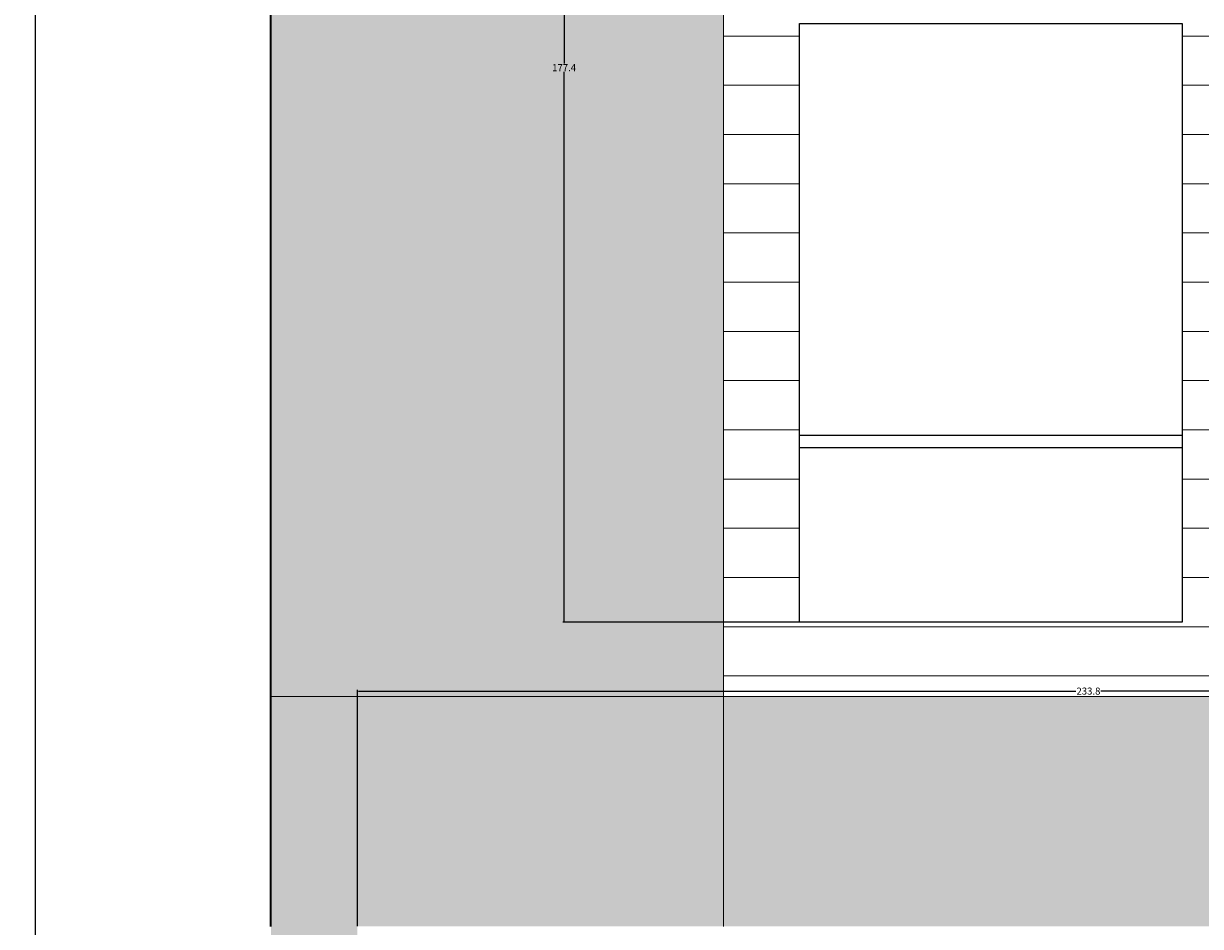
# Model space of a CAD drawing. Units: inches. Extents: x 8 to 634, y 41 to 867.
# Tile 3 of 21: x 8 to 196, y 236 to 380. Entities that reach past the tile are written whole.
import ezdxf

# ---------------------------------------------------------------- set-up
doc = ezdxf.new("R2010")
doc.units = ezdxf.units.IN
doc.header["$MEASUREMENT"] = 0
for name, color, linetype, lineweight in [('A-ANNO-DIMS', 2, 'Continuous', 18), ('A-GLAZ', 4, 'Continuous', 25), ('A-WALL', 7, 'Continuous', 35), ('A-WALL-PANL', 7, 'Continuous', 18), ('A-WALL-PATT', 8, 'Continuous', 9)]:
    doc.layers.add(name, color=color, linetype=linetype, lineweight=lineweight)
doc.styles.get("Standard").update_dxf_attribs({"font": 'arial.ttf'})
doc.dimstyles.get("Standard").update_dxf_attribs({"dimtxt": 1.125, "dimasz": 0.18, "dimexe": 0.18, "dimexo": 0.0625, "dimgap": 0.09, "dimtad": 0, "dimtih": 1, "dimtoh": 1, "dimdec": 4, "dimzin": 0, "dimdsep": 46, "dimlunit": 4, "dimtxsty": 'Standard', "dimcen": 0.09, "dimadec": 0, "dimazin": 0, "dimtfac": 1, "dimtdec": 4, "dimtofl": 0, "dimtmove": 0, "dimatfit": 3, "dimfxl": 1, "dimtolj": 1, "dimtzin": 0, "dimarcsym": 0})

# ---------------------------------------------------------------- blocks, each defined once
blk = doc.blocks.new('WIN-DOUBLE-RAIL')
for p, q in [((0, 29.93), (61.23, 29.93)), ((0, 27.93), (61.23, 27.93))]:
    blk.add_line(p, q)
blk.add_lwpolyline([(0, 95.77), (61.23, 95.77), (61.23, 0), (0, 0)], close=True)
blk = doc.blocks.new('*D20')
at = {"layer": 'A-ANNO-DIMS', "color": 0, "lineweight": -2, "transparency": 16777216}
for p, q in [((144.29, 828.98), (9.51, 828.98)), ((9.69, 828.8), (9.69, 454.93)), ((9.69, 79.74), (9.69, 453.6)), ((47.28, 79.56), (9.51, 79.56))]:
    blk.add_line(p, q, dxfattribs=at)
at = {"layer": 'A-ANNO-DIMS', "color": 0, "transparency": 16777216}
for points in [[(9.66, 828.8), (9.72, 828.8), (9.69, 828.98)], [(9.66, 79.74), (9.72, 79.74), (9.69, 79.56)]]:
    blk.add_solid(points, dxfattribs=at)
at = {"layer": 'Defpoints', "color": 0, "transparency": 16777216}
for p in [(9.69, 828.98), (144.36, 828.98), (47.34, 79.56)]:
    blk.add_point(p, dxfattribs=at)
at = {"layer": 'A-ANNO-DIMS', "color": 0, "transparency": 16777216, "insert": (9.69, 454.27), "char_height": 1.125, "attachment_point": 5}
blk.add_mtext('\\A1;749.4', dxfattribs=at)
blk = doc.blocks.new('*D43')
at = {"layer": 'A-ANNO-DIMS', "color": 0, "lineweight": -2, "transparency": 16777216}
for p, q in [((131.81, 461.65), (94.05, 461.65)), ((94.23, 461.47), (94.23, 373.6)), ((94.23, 284.42), (94.23, 372.29)), ((131.81, 284.24), (94.05, 284.24))]:
    blk.add_line(p, q, dxfattribs=at)
at = {"layer": 'A-ANNO-DIMS', "color": 0, "transparency": 16777216}
for points in [[(94.2, 461.47), (94.26, 461.47), (94.23, 461.65)], [(94.2, 284.42), (94.26, 284.42), (94.23, 284.24)]]:
    blk.add_solid(points, dxfattribs=at)
at = {"layer": 'Defpoints', "color": 0, "transparency": 16777216}
for p in [(94.23, 461.65), (131.88, 461.65), (131.88, 284.24)]:
    blk.add_point(p, dxfattribs=at)
at = {"layer": 'A-ANNO-DIMS', "color": 0, "transparency": 16777216, "insert": (94.23, 372.95), "char_height": 1.125, "attachment_point": 5}
blk.add_mtext('\\A1;177.4', dxfattribs=at)
blk = doc.blocks.new('*D65')
at = {"layer": 'A-ANNO-DIMS', "color": 0, "lineweight": -2, "transparency": 16777216}
for p, q in [((61.18, 235.62), (61.18, 273.39)), ((61.36, 273.21), (176.09, 273.21)), ((294.82, 273.21), (180.09, 273.21)), ((295, 235.62), (295, 273.39))]:
    blk.add_line(p, q, dxfattribs=at)
at = {"layer": 'A-ANNO-DIMS', "color": 0, "transparency": 16777216}
for points in [[(61.36, 273.24), (61.36, 273.18), (61.18, 273.21)], [(294.82, 273.24), (294.82, 273.18), (295, 273.21)]]:
    blk.add_solid(points, dxfattribs=at)
at = {"layer": 'Defpoints', "color": 0, "transparency": 16777216}
for p in [(295, 273.21), (61.18, 235.56), (295, 235.56)]:
    blk.add_point(p, dxfattribs=at)
at = {"layer": 'A-ANNO-DIMS', "color": 0, "transparency": 16777216, "insert": (178.09, 273.21), "char_height": 1.125, "attachment_point": 5}
blk.add_mtext('\\A1;233.8', dxfattribs=at)

msp = doc.modelspace()

# ---------------------------------------------------------------- hatches: boundary and pattern name
at = {"layer": 'A-WALL-PATT', "transparency": 33554687}
h = msp.add_hatch(dxfattribs=at)
h.set_pattern_fill('AR-CONC', color=256, scale=3.2)
h.paths.add_polyline_path([(119.7065, 697.6655), (47.3401, 697.6655), (47.3401, 569.1705), (119.7065, 569.1705)])
h.paths.add_polyline_path([(202.1558, 697.6655), (119.7065, 697.6655), (119.7065, 569.1705), (202.1558, 569.1705)])
h.paths.add_polyline_path([(284.6051, 697.6655), (202.1558, 697.6655), (202.1558, 569.1705), (284.6051, 569.1705)])
h.paths.add_polyline_path([(119.7065, 569.1705), (47.3401, 569.1705), (47.3401, 523.5555), (47.3401, 449.7533), (119.7065, 449.7533)])
h.paths.add_polyline_path([(342.6544, 682.1444), (360.785, 697.6655), (284.6051, 697.6655), (284.6051, 569.1705), (342.6544, 569.1705)])
h.paths.add_polyline_path([(342.6544, 569.1705), (284.6051, 569.1705), (284.6051, 449.7533), (342.6544, 449.7533)])
h.paths.add_polyline_path([(418.2881, 691.978), (418.2881, 697.6655), (360.785, 697.6655), (360.785, 569.1705), (418.2881, 569.1705)])
h.paths.add_polyline_path([(418.2881, 569.1705), (360.785, 569.1705), (360.785, 523.5555), (360.785, 449.7533), (418.2881, 449.7533)])
h.paths.add_polyline_path([(594.3501, 697.6655), (539.0002, 697.6655), (539.0002, 691.978), (539.0002, 569.1705), (594.3501, 569.1705)])
h.paths.add_polyline_path([(594.3501, 523.5555), (594.3501, 569.1705), (539.0002, 569.1705), (539.0002, 451.6305), (594.3501, 451.6305)])
h.paths.add_polyline_path([(594.3501, 451.6305), (539.0002, 451.6305), (539.0002, 391.7598), (594.3501, 391.7598)])
h.paths.add_polyline_path([(594.3501, 391.7598), (539.0002, 391.7598), (539.0002, 276.166), (594.3501, 276.166)])
h.paths.add_polyline_path([(418.2881, 449.7533), (360.785, 449.7533), (360.785, 391.7598), (418.2881, 391.7598)])
h.paths.add_polyline_path([(342.6544, 449.7533), (284.6051, 449.7533), (284.6051, 391.7598), (342.6544, 391.7598)])
h.paths.add_polyline_path([(342.6544, 391.7598), (284.6051, 391.7598), (284.6051, 272.3426), (342.6544, 272.3426)])
h.paths.add_polyline_path([(418.2881, 391.7598), (360.785, 391.7598), (360.785, 272.3426), (418.2881, 272.3426)])
h.paths.add_polyline_path([(418.2881, 272.3426), (360.785, 272.3426), (360.785, 235.5555), (418.2881, 235.5555)])
h.paths.add_polyline_path([(342.6544, 272.3426), (284.6051, 272.3426), (284.6051, 235.5555), (295.0049, 235.5555), (342.6544, 235.5555)])
h.paths.add_polyline_path([(594.3501, 276.166), (539.0002, 276.166), (539.0002, 228.4951), (594.3501, 228.4951)])
h.paths.add_polyline_path([(594.3501, 228.4951), (539.0002, 228.4951), (539.0002, 91.5417), (594.3501, 91.5417)])
h.paths.add_polyline_path([(418.2881, 235.5555), (360.785, 235.5555), (360.785, 91.5417), (418.2881, 91.5417)])
h.paths.add_polyline_path([(284.6051, 272.3426), (119.7065, 272.3426), (119.7065, 235.5555), (284.6051, 235.5555)])
h.paths.add_polyline_path([(119.7065, 272.3426), (47.3401, 272.3426), (47.3401, 235.5555), (47.3401, 91.5555), (63.5448, 91.5555), (63.5448, 227.8036), (268.998, 227.8036), (268.998, 91.5555), (295.0049, 91.5555), (295.0049, 222.583), (271.9787, 222.583), (271.9787, 229.0481), (62.4019, 229.0481), (62.4019, 222.583), (61.1827, 222.583), (61.1827, 235.5555), (119.7065, 235.5555)])
h.paths.add_polyline_path([(119.7065, 391.7598), (47.3401, 391.7598), (47.3401, 379.5555), (47.3401, 272.3426), (119.7065, 272.3426)])
h.paths.add_polyline_path([(119.7065, 449.7533), (47.3401, 449.7533), (47.3401, 391.7598), (119.7065, 391.7598)])
h.paths.add_polyline_path([(202.1558, 449.7533), (119.7065, 449.7533), (119.7065, 391.7598), (202.1558, 391.7598)])
h.paths.add_polyline_path([(284.6051, 449.7533), (202.1558, 449.7533), (202.1558, 391.7598), (284.6051, 391.7598)])
at = {"layer": 'A-WALL-PATT', "transparency": 33554681}
h = msp.add_hatch(dxfattribs=at)
h.set_pattern_fill('ANSI31', color=256, scale=63, angle=135)
h.paths.add_polyline_path([(284.6051, 391.7598), (119.7065, 391.7598), (119.7065, 272.3426), (284.6051, 272.3426)])
h.paths.add_polyline_path([(193.1116, 284.2398), (131.8771, 284.2398), (131.8771, 380.0085), (193.1116, 380.0085)], flags=16)
h.paths.add_polyline_path([(207.7547, 380.0085), (268.9893, 380.0085), (268.9893, 284.2398), (207.7547, 284.2398)], flags=16)
h.paths.add_polyline_path([(342.6544, 235.5555), (295.0049, 235.5555), (295.0049, 91.5417), (342.6544, 91.5417)])

# ---------------------------------------------------------------- linework, layer by layer
at = {"layer": 'A-WALL'}
for p, q in [((47.3401, 379.5555), (47.3401, 523.5555)), ((47.3401, 235.5555), (47.3401, 379.5555)), ((47.3401, 379.5555), (47.3401, 379.5555))]:
    msp.add_line(p, q, dxfattribs=at)
at = {"layer": 'A-WALL-PANL'}
for q in [(47.3401, 272.3426), (119.7065, 235.5555)]:
    msp.add_line((119.7065, 272.3426), q, dxfattribs=at)
msp.add_lwpolyline([(119.7065, 391.7598), (284.6051, 391.7598), (284.6051, 272.3426), (119.7065, 272.3426)], close=True, dxfattribs=at)

# ---------------------------------------------------------------- block references
at = {"layer": 'A-GLAZ'}
msp.add_blockref('WIN-DOUBLE-RAIL', (131.877, 284.24), dxfattribs=at)

# ---------------------------------------------------------------- dimensions: what is measured, and where the dimension line sits
at = {"layer": 'A-ANNO-DIMS'}
for base, p1, p2, picture, middle in [((9.6901, 828.9821), (47.3401, 79.5555), (144.3564, 828.9821), '*D20', (9.6901, 454.2688)), ((94.2271, 461.6505), (131.8771, 284.2398), (131.8771, 461.6505), '*D43', (94.2271, 372.9452))]:
    dim = msp.add_linear_dim(base=base, p1=p1, p2=p2, angle=90, dimstyle='Standard', override={"dimdec": 1, "dimlfac": 1, "dimrnd": 0, "dimzin": 0, "dimdsep": 46, "dimlunit": 2}, dxfattribs=at)
    dim.commit()
    dim.dimension.update_dxf_attribs({"geometry": picture, "text_midpoint": middle})
dim = msp.add_linear_dim(base=(295.0049, 273.2055), p1=(61.1827, 235.5555), p2=(295.0049, 235.5555), dimstyle='Standard', override={"dimdec": 1, "dimlfac": 1, "dimrnd": 0, "dimzin": 0, "dimdsep": 46, "dimlunit": 2}, dxfattribs=at)
dim.commit()
dim.dimension.update_dxf_attribs({"geometry": '*D65', "text_midpoint": (178.0938, 273.2055)})

doc.saveas('drawing.dxf')
